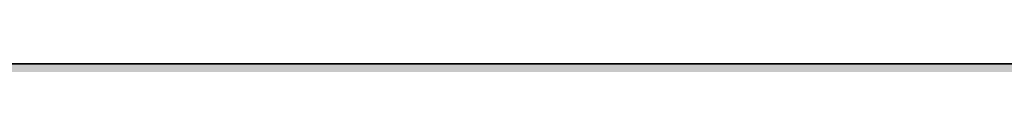
# Model space of a CAD drawing. Units: inches. Extents: x 2091 to 2899, y 967 to 2217.
# Tile 59 of 256: x 2212.20615 to 2212.29411, y 1099.91903 to 1099.91906. Entities that reach past the tile are written whole.
import ezdxf

# ---------------------------------------------------------------- set-up
doc = ezdxf.new("R2010")
doc.units = ezdxf.units.IN
doc.layers.add('A-WALL-PATT', color=141, linetype='Continuous', lineweight=13, true_color=0xadddf7)
doc.layers.add('L-SITE-WALL', color=7, linetype='Continuous', lineweight=35)

msp = doc.modelspace()

# ---------------------------------------------------------------- hatches: boundary and pattern name
at = {"layer": 'A-WALL-PATT'}
h = msp.add_hatch(color=256, dxfattribs=at)
h.dxf.hatch_style = 1
h.paths.add_polyline_path([(2212.143603, 1941.419059), (2387.643603, 1941.419059), (2387.643603, 1824.419059), (2392.143603, 1824.419059), (2392.143603, 1941.419059), (2609.643603, 1941.419059), (2609.643603, 1825.919059), (2614.143603, 1825.919059), (2614.143603, 1941.419059), (2794.143603, 1941.419059), (2794.143603, 1928.762166), (2803.143603, 1928.762166), (2803.143603, 2050.919059), (2203.143603, 2050.919059), (2203.143603, 1900.757859), (2212.143603, 1900.757859)])
h.paths.add_polyline_path([(2212.143603, 1945.919059), (2212.143603, 2041.919059), (2794.143603, 2041.919059), (2794.143603, 1945.919059), (2402.248245, 1945.919059), (2401.102434, 1945.775832), (2398.702434, 1945.775832)], flags=16)
h.paths.add_polyline_path([(2230.229861, 1948.062793), (2227.349861, 1949.502793), (2225.909861, 1951.902793), (2223.989861, 1952.862793), (2223.029861, 1955.262793), (2222.069861, 1959.582793), (2222.069861, 1963.422793), (2223.029861, 1965.662793), (2223.989861, 1965.342793), (2225.58591, 1963.860747), (2226.911533, 1964.957259), (2226.948861, 1965.938793), (2227.778319, 1966.952143), (2228.199916, 1968.878704), (2230.709861, 1964.862793), (2233.589861, 1966.302793), (2233.607309, 1966.331873), (2233.772659, 1964.938205), (2234.633802, 1963.676473), (2235.029861, 1963.902793), (2236.282035, 1965.572358), (2235.989861, 1962.942793), (2237.954512, 1957.540002), (2238.389861, 1957.902793), (2239.215861, 1960.305793), (2238.654565, 1966.38496), (2238.692792, 1966.438069), (2238.840578, 1967.499707), (2238.780291, 1967.687486), (2238.880538, 1967.786763), (2238.666861, 1966.251793), (2239.215861, 1960.305793), (2238.389861, 1957.902793), (2236.949861, 1956.702793), (2234.549861, 1949.982793)], flags=0)
h.paths.add_polyline_path([(2278.011974, 1948.062793), (2276.496427, 1947.873349), (2275.849833, 1947.688608), (2274.651974, 1947.102793)], flags=0)
h.paths.add_polyline_path([(2269.851974, 1955.742793), (2268.276176, 1956.629329), (2270.867302, 1956.348398), (2269.371974, 1958.142793), (2268.714964, 1959.192325), (2270.569833, 1958.728608), (2268.580725, 1961.906087), (2270.811974, 1960.891883), (2270.811974, 1963.422793), (2271.393315, 1964.779256), (2270.291762, 1966.156196), (2271.771974, 1965.662793), (2272.141387, 1966.524757), (2273.929833, 1965.928608), (2275.630385, 1968.054299), (2276.331938, 1966.72186), (2276.520431, 1966.952143), (2276.942029, 1968.878704), (2277.734293, 1967.611082), (2278.139888, 1969.46452), (2279.659124, 1967.033742), (2280.411974, 1966.782793), (2280.949302, 1967.588785), (2281.609833, 1967.368608), (2282.133266, 1968.153758), (2282.349235, 1966.333445), (2282.349849, 1966.332585), (2283.40755, 1968.09542), (2283.712631, 1965.52402), (2284.320221, 1964.633789), (2284.511809, 1964.889239), (2284.234974, 1965.704793), (2284.500472, 1967.318958), (2284.907944, 1965.41742), (2285.396313, 1966.068579), (2285.432833, 1966.290608), (2285.473338, 1966.171279), (2286.353919, 1967.345387), (2286.222007, 1966.158173), (2287.663492, 1968.080154), (2287.713974, 1968.442793), (2288.481599, 1969.016679), (2288.573993, 1968.728897), (2288.917461, 1969.06904), (2288.606833, 1966.837608), (2288.928726, 1963.35131), (2288.934974, 1963.356793), (2288.929731, 1963.340422), (2289.015281, 1962.413869), (2290.111223, 1963.875126), (2290.132833, 1963.942608), (2290.217672, 1964.017058), (2290.111223, 1963.875126), (2289.155833, 1960.891608), (2288.594036, 1959.257227), (2288.571974, 1959.102793), (2289.531974, 1960.542793), (2290.011974, 1962.462793), (2290.19184, 1962.642659), (2289.769833, 1959.688608), (2286.889833, 1957.288608), (2284.489833, 1950.568608), (2283.314658, 1950.046308), (2283.291974, 1949.982793), (2280.290059, 1948.648608), (2281.129833, 1948.648608), (2282.569833, 1948.168608), (2283.204726, 1948.062793), (2278.971974, 1948.062793), (2276.091974, 1949.502793), (2274.651974, 1951.902793), (2272.731974, 1952.862793)], flags=0)
h.paths.add_polyline_path([(2271.158868, 1958.021765), (2272.969833, 1955.848608), (2272.009833, 1960.168608), (2272.009833, 1964.008608), (2272.624426, 1965.442658), (2274.328023, 1963.860747), (2275.653646, 1964.957259), (2275.637743, 1964.53909), (2277.412231, 1966.006888), (2277.032974, 1965.156793), (2276.829924, 1964.975597), (2276.766012, 1963.295014), (2277.449635, 1962.66022), (2279.451974, 1964.862793), (2282.331974, 1966.302793), (2283.529833, 1966.888608), (2283.294512, 1966.770948), (2283.912993, 1963.8847), (2284.899249, 1964.448275), (2284.731974, 1962.942793), (2286.696625, 1957.540002), (2287.131974, 1957.902793), (2287.541913, 1959.095388), (2287.779395, 1958.442311), (2285.682738, 1956.695097), (2285.876503, 1959.795336), (2284.731974, 1962.942793), (2284.899249, 1964.448275), (2283.912993, 1963.8847), (2284.223833, 1962.434116), (2283.424365, 1963.605484), (2281.609833, 1962.568608), (2281.129833, 1960.168608), (2282.089833, 1956.328608), (2283.049833, 1952.968608), (2282.569833, 1950.568608), (2280.169833, 1948.648608), (2279.883316, 1948.791867), (2278.971974, 1948.062793), (2278.971974, 1949.022793), (2278.672313, 1949.397368), (2277.289833, 1950.088608), (2275.849833, 1952.488608), (2273.929833, 1953.448608), (2272.489833, 1954.888608), (2271.921647, 1954.888608), (2271.771974, 1955.262793)], flags=0)
h.paths.add_polyline_path([(2311.994146, 1955.742793), (2312.062717, 1955.674221), (2312.0551, 1955.7085)], flags=0)
h.paths.add_polyline_path([(2331.956146, 1963.951793), (2333.396146, 1965.391793), (2331.077146, 1963.356793), (2330.998603, 1963.111517)], flags=0)
h.paths.add_polyline_path([(2310.554146, 1954.302793), (2307.039807, 1956.279943), (2310.762903, 1955.876284), (2312.474146, 1953.822793), (2313.434146, 1951.422793), (2315.354146, 1950.462793), (2316.794146, 1948.062793), (2317.466146, 1947.726793), (2319.368691, 1947.964611), (2317.754146, 1949.982793), (2317.569531, 1950.610485), (2316.794146, 1951.902793), (2314.874146, 1952.862793), (2313.914146, 1955.262793), (2311.514146, 1958.142793), (2309.375489, 1961.559168), (2311.514146, 1960.337078), (2311.514146, 1961.982793), (2310.604672, 1963.119635), (2311.726605, 1962.47853), (2312.418332, 1964.09256), (2312.255964, 1964.29552), (2313.194146, 1963.982793), (2313.914146, 1965.662793), (2314.646778, 1965.418582), (2315.354146, 1966.302793), (2316.794146, 1967.742793), (2316.157435, 1966.946904), (2317.034111, 1965.28186), (2317.222604, 1965.512143), (2317.777048, 1968.045771), (2318.474111, 1966.72186), (2318.662604, 1966.952143), (2319.084201, 1968.878704), (2321.207049, 1965.482147), (2322.161419, 1966.913702), (2322.554146, 1966.782793), (2322.785988, 1967.130555), (2322.881646, 1966.324293), (2323.312041, 1965.72174), (2323.651289, 1965.891364), (2324.3965, 1967.133382), (2324.656945, 1964.938205), (2324.971986, 1964.476611), (2325.38728, 1967.001499), (2325.940813, 1964.418348), (2327.228929, 1966.135836), (2327.16632, 1965.572358), (2328.059139, 1966.762783), (2328.224576, 1966.247486), (2329.667971, 1967.67691), (2329.664576, 1967.687486), (2329.764823, 1967.786763), (2329.551146, 1966.251793), (2330.100146, 1960.305793), (2329.332814, 1958.07347), (2329.313065, 1957.935225), (2329.634146, 1958.202793), (2330.234146, 1959.102793), (2330.714146, 1961.022793), (2331.034146, 1961.342793), (2330.714146, 1959.102793), (2329.634146, 1958.202793), (2329.274146, 1957.662793), (2327.712112, 1956.361098), (2325.434146, 1949.982793), (2324.333769, 1949.493736), (2323.994146, 1948.542793), (2319.674146, 1946.622793), (2316.794146, 1948.062793), (2315.354146, 1950.462793), (2313.434146, 1951.422793)], flags=0)
h.paths.add_polyline_path([(2321.335684, 1947.952023), (2321.114146, 1948.062793), (2321.114146, 1949.022793), (2319.194146, 1951.422793), (2316.794146, 1959.582793), (2316.663237, 1959.582793), (2315.354146, 1958.142793), (2314.394146, 1958.142793), (2313.148303, 1958.709085), (2312.954146, 1959.582793), (2312.954146, 1960.891883), (2315.834146, 1959.582793), (2316.663237, 1959.582793), (2317.314709, 1960.299412), (2315.030195, 1962.420747), (2316.355818, 1963.517259), (2316.372337, 1963.951615), (2316.470195, 1963.860747), (2317.795818, 1964.957259), (2317.755219, 1963.889687), (2319.175146, 1965.156793), (2319.498407, 1965.881372), (2321.114146, 1965.342793), (2323.235885, 1962.372358), (2325.686349, 1963.772623), (2325.542789, 1962.480576), (2325.198783, 1963.494014), (2324.47851, 1963.082429), (2324.926005, 1960.994116), (2324.078087, 1962.236473), (2322.414791, 1961.286018), (2322.074146, 1959.582793), (2323.034146, 1955.742793), (2323.994146, 1952.382793), (2323.514146, 1949.982793), (2322.142717, 1948.88565), (2322.074146, 1948.542793)], flags=0)
h.paths.add_polyline_path([(2320.207479, 1963.337459), (2320.154146, 1963.422793), (2320.394146, 1963.542793)], flags=0)
h.paths.add_polyline_path([(2353.850527, 1965.8105), (2354.030527, 1965.7505), (2354.330527, 1966.4505), (2354.330527, 1966.9305)], flags=0)
h.paths.add_polyline_path([(2359.020582, 1969.026412), (2359.098382, 1968.901932), (2359.233527, 1969.5195), (2359.233527, 1969.9995)], flags=0)
h.paths.add_polyline_path([(2358.256694, 1966.681672), (2357.983601, 1966.348035), (2358.211267, 1966.146175), (2358.410492, 1966.389568)], flags=0)
h.paths.add_polyline_path([(2357.768473, 1966.058778), (2357.7322, 1965.104967), (2357.751047, 1965.120556), (2357.769527, 1965.6065), (2357.769527, 1966.057843)], flags=0)
h.paths.add_polyline_path([(2359.111527, 1965.3045), (2359.111527, 1964.8245), (2359.844527, 1966.4675), (2359.844527, 1966.9475)], flags=0)
h.paths.add_polyline_path([(2360.223684, 1966.621449), (2360.698527, 1969.3625), (2360.698527, 1969.8425), (2360.210527, 1967.0255), (2360.210527, 1966.6425)], flags=0)
h.paths.add_polyline_path([(2363.450527, 1967.8905), (2363.450527, 1968.3705), (2362.490527, 1966.9305), (2362.656045, 1966.698776)], flags=0)
h.paths.add_polyline_path([(2364.475523, 1966.078826), (2365.850527, 1968.3705), (2365.850527, 1968.8505), (2364.427975, 1966.479581)], flags=0)
h.paths.add_polyline_path([(2366.313527, 1965.8525), (2366.366709, 1965.695829), (2366.802527, 1968.3455), (2366.802527, 1968.8255)], flags=0)
h.paths.add_polyline_path([(2367.16531, 1965.803544), (2367.290527, 1966.9305), (2367.290527, 1967.4105), (2367.102701, 1965.720066)], flags=0)
h.paths.add_polyline_path([(2370.036527, 1959.9735), (2371.013527, 1963.0245), (2371.013527, 1963.5045), (2370.036527, 1960.4535)], flags=0)
h.paths.add_polyline_path([(2371.610527, 1960.2105), (2372.570527, 1961.6505), (2372.570527, 1962.1305), (2371.802527, 1960.9785)], flags=0)
h.paths.add_polyline_path([(2350.873666, 1956.005086), (2351.930527, 1955.8905), (2354.490527, 1953.3305), (2353.850527, 1954.9305), (2351.450527, 1957.8105), (2347.935527, 1963.4255), (2347.935527, 1963.9055), (2351.450527, 1958.2905), (2353.705073, 1955.585046), (2352.890527, 1959.2505), (2352.890527, 1959.7305), (2352.890527, 1961.924786), (2356.730527, 1959.7305), (2358.454471, 1961.626838), (2354.810527, 1965.0105), (2355.030855, 1965.28591), (2358.691091, 1961.88712), (2361.530527, 1965.0105), (2364.376495, 1966.433484), (2364.524394, 1965.186911), (2365.454468, 1963.824181), (2365.881073, 1964.067955), (2365.370527, 1966.4505), (2365.370527, 1966.9305), (2366.810527, 1960.2105), (2366.810527, 1959.7305), (2366.388709, 1952.981409), (2367.770527, 1956.8505), (2368.641225, 1957.576082), (2366.810527, 1962.6105), (2366.810527, 1963.0905), (2368.775179, 1957.68771), (2369.210527, 1958.0505), (2370.001592, 1960.351867), (2369.475232, 1966.052668), (2369.513458, 1966.105777), (2369.514173, 1966.110912), (2369.475232, 1966.532668), (2369.513458, 1966.585777), (2369.614635, 1967.312591), (2369.182527, 1968.6585), (2369.182527, 1969.1385), (2369.600957, 1967.835194), (2369.701204, 1967.934471), (2369.717947, 1968.054743), (2370.145176, 1968.374145), (2369.778707, 1968.011224), (2369.701204, 1967.454471), (2370.468161, 1968.214004), (2369.674936, 1967.265771), (2369.514173, 1966.110912), (2370.036527, 1960.4535), (2370.036527, 1959.9735), (2369.441756, 1958.243191), (2370.650527, 1959.2505), (2371.045821, 1962.017559), (2371.130527, 1962.1305), (2370.650527, 1958.7705), (2367.770527, 1956.3705), (2365.370527, 1949.6505), (2362.079099, 1948.187643), (2363.450527, 1947.7305), (2361.050527, 1947.7305), (2360.090527, 1947.7305), (2357.103861, 1947.357167), (2360.090527, 1948.2105), (2358.170527, 1949.1705), (2356.730527, 1951.5705), (2354.810527, 1952.5305), (2351.930527, 1955.4105)], flags=0)
h.paths.add_polyline_path([(2361.050527, 1948.6905), (2359.130527, 1951.0905), (2356.730527, 1959.2505), (2355.770527, 1959.2505), (2352.890527, 1960.559591), (2352.890527, 1961.444786), (2355.890527, 1959.7305), (2356.730527, 1959.7305), (2356.837194, 1959.367834), (2361.530527, 1964.5305), (2363.248422, 1965.389448), (2364.92531, 1963.041805), (2362.490527, 1961.6505), (2362.063861, 1959.517167), (2362.970527, 1955.8905), (2363.930527, 1952.5305), (2363.930527, 1952.0505), (2363.450527, 1949.6505), (2361.050527, 1947.7305)], flags=0)
h.paths.add_polyline_path([(2359.130527, 1951.5705), (2359.290527, 1951.3705), (2361.050527, 1954.4505), (2361.050527, 1954.9305)], flags=0)
h.paths.add_polyline_path([(2357.219527, 1966.5455), (2356.792527, 1968.8145), (2356.792527, 1969.2945), (2357.219527, 1967.0255)], flags=0)
h.paths.add_polyline_path([(2361.050527, 1954.4505), (2361.530527, 1958.7705), (2361.530527, 1959.2505), (2361.050527, 1954.9305)], flags=0)
h.paths.add_polyline_path([(2402.548287, 1948.486076), (2402.302434, 1948.415832), (2402.590434, 1948.415832)], flags=0)
h.paths.add_polyline_path([(2394.142434, 1956.095832), (2395.685052, 1954.553214), (2396.720495, 1953.970679), (2396.062434, 1955.615832), (2395.241381, 1956.601096), (2395.878904, 1956.441715), (2395.102434, 1959.935832), (2395.102434, 1963.775832), (2396.062434, 1966.015832), (2397.022434, 1965.695832), (2398.618483, 1964.213787), (2399.944106, 1965.310299), (2399.981434, 1966.291832), (2400.810891, 1967.305183), (2401.232489, 1969.231744), (2403.537949, 1965.543008), (2403.941984, 1967.389316), (2404.702434, 1967.135832), (2405.460328, 1966.07478), (2406.622434, 1966.655832), (2406.639882, 1966.684913), (2406.805232, 1965.291245), (2406.925694, 1965.114746), (2407.342434, 1964.975832), (2407.874326, 1965.77367), (2408.1691, 1964.398055), (2409.314608, 1965.925398), (2409.217458, 1965.051054), (2409.445232, 1963.131245), (2410.306374, 1961.869513), (2410.702434, 1962.095832), (2411.442269, 1963.082279), (2411.165434, 1963.897832), (2411.616426, 1966.639757), (2411.725365, 1966.791109), (2411.873151, 1967.852747), (2411.812864, 1968.040526), (2411.913111, 1968.139803), (2411.699434, 1966.604832), (2412.248434, 1960.658832), (2413.225434, 1963.709832), (2414.3779, 1964.72116), (2414.513151, 1965.692747), (2414.452864, 1965.880526), (2414.553111, 1965.979803), (2414.3779, 1964.72116), (2414.519817, 1964.845697), (2414.365365, 1964.631109), (2414.339434, 1964.444832), (2414.888434, 1958.498832), (2414.062434, 1956.095832), (2412.622434, 1954.895832), (2410.17137, 1948.032854), (2410.016719, 1948.084404), (2405.902434, 1946.255832), (2405.902434, 1947.215832), (2405.204252, 1948.08856), (2404.222434, 1948.415832), (2403.262434, 1948.415832), (2400.382434, 1949.855832), (2399.662434, 1951.055832), (2397.982434, 1952.735832), (2397.022434, 1953.215832), (2395.685052, 1954.553214), (2392.656776, 1956.256908)], flags=0)
h.paths.add_polyline_path([(2409.08565, 1964.407441), (2409.130363, 1964.275715), (2409.262434, 1964.495832)], flags=0)
h.paths.add_polyline_path([(2397.742434, 1961.615832), (2398.702434, 1963.855832), (2399.662434, 1963.535832), (2401.426563, 1965.740994), (2401.791415, 1966.5588), (2402.071434, 1965.070832), (2402.835507, 1964.393367), (2403.262398, 1964.9149), (2403.338119, 1964.771086), (2402.615516, 1963.976223), (2402.498612, 1960.902238), (2403.542997, 1959.932452), (2404.413203, 1960.889679), (2404.702434, 1962.335832), (2407.916347, 1964.172354), (2409.520211, 1961.926944), (2410.987085, 1957.893042), (2411.422434, 1958.255832), (2412.047964, 1960.075625), (2412.410341, 1959.079088), (2411.675621, 1958.466821), (2411.662434, 1958.255832), (2411.62607, 1958.425529), (2409.982434, 1957.055832), (2407.582434, 1950.335832), (2403.262434, 1948.415832), (2403.262434, 1949.375832), (2401.342434, 1951.775832), (2399.416508, 1958.323981), (2397.742434, 1959.084923), (2397.742434, 1959.970118), (2397.102434, 1960.335832), (2397.742434, 1960.044923)], flags=0)
h.paths.add_polyline_path([(2405.902434, 1952.975832), (2405.950434, 1953.407832), (2406.016719, 1953.175832)], flags=0)
h.paths.add_polyline_path([(2449.817778, 1967.114014), (2449.752323, 1967.135832), (2449.793703, 1967.077901)], flags=0)
h.paths.add_polyline_path([(2451.697696, 1966.61812), (2451.740895, 1966.690118), (2451.692051, 1966.665696)], flags=0)
h.paths.add_polyline_path([(2454.343628, 1965.737572), (2455.752323, 1967.615832), (2455.992323, 1968.095832), (2454.364497, 1965.925398)], flags=0)
h.paths.add_polyline_path([(2457.547323, 1968.863832), (2457.787323, 1969.343832), (2457.054323, 1968.795832), (2457.007622, 1968.460345)], flags=0)
h.paths.add_polyline_path([(2456.921784, 1967.856662), (2456.802238, 1968.229016), (2456.723, 1967.659803)], flags=0)
h.paths.add_polyline_path([(2457.302323, 1967.376832), (2457.542323, 1967.856832), (2456.810323, 1966.839832), (2456.740516, 1966.700218), (2456.749021, 1966.608105)], flags=0)
h.paths.add_polyline_path([(2458.275323, 1963.709832), (2458.155343, 1963.335153), (2460.354323, 1965.264832), (2460.594323, 1965.744832)], flags=0)
h.paths.add_polyline_path([(2458.392323, 1962.815832), (2458.364088, 1962.618185), (2459.592323, 1964.255832), (2459.832323, 1964.735832)], flags=0)
h.paths.add_polyline_path([(2459.352323, 1962.815832), (2459.272323, 1962.495832), (2460.072323, 1963.295832), (2460.312323, 1963.775832)], flags=0)
h.paths.add_polyline_path([(2458.680323, 1960.607832), (2458.632323, 1960.415832), (2459.592323, 1961.855832), (2459.832323, 1962.335832)], flags=0)
h.paths.add_polyline_path([(2437.83817, 1956.24265), (2439.192323, 1956.095832), (2441.352323, 1953.935832), (2440.872323, 1955.135832), (2438.472323, 1958.015832), (2438.071563, 1958.656023), (2438.712323, 1958.495832), (2440.639596, 1956.183105), (2439.912323, 1959.455832), (2439.912323, 1963.295832), (2441.352323, 1966.655832), (2441.592323, 1967.135832), (2441.112323, 1966.015832), (2442.072323, 1965.695832), (2443.988993, 1968.09167), (2444.241323, 1966.750832), (2444.916801, 1966.15192), (2445.676574, 1967.080136), (2446.255323, 1969.724832), (2446.495323, 1970.204832), (2446.282379, 1969.231744), (2447.362672, 1967.503275), (2447.720323, 1969.567832), (2447.960323, 1970.047832), (2447.48548, 1967.306781), (2448.792323, 1965.215832), (2448.472323, 1964.863832), (2448.552323, 1964.735832), (2451.452051, 1966.185696), (2451.615122, 1964.811245), (2452.307917, 1963.796172), (2453.234505, 1964.325651), (2454.072323, 1960.415832), (2453.628687, 1953.317651), (2454.792323, 1956.575832), (2455.032323, 1957.055832), (2455.718835, 1957.627926), (2453.832323, 1962.815832), (2453.940966, 1963.793615), (2453.335323, 1965.577832), (2453.824323, 1968.550832), (2454.064323, 1969.030832), (2453.575323, 1966.057832), (2454.040333, 1964.687919), (2453.832323, 1962.815832), (2455.718835, 1957.627926), (2456.367207, 1958.168235), (2457.058323, 1960.178832), (2457.298323, 1960.658832), (2456.472323, 1958.255832), (2457.717729, 1959.29367), (2457.672323, 1958.975832), (2454.889951, 1956.657188), (2453.614142, 1953.084923), (2453.592323, 1952.735832), (2453.352323, 1952.255832), (2453.359596, 1952.372196), (2452.632323, 1950.335832), (2452.392323, 1949.855832), (2449.203752, 1948.43869), (2450.712323, 1947.935832), (2448.072323, 1947.935832), (2447.112323, 1947.935832), (2444.552323, 1947.615832), (2447.199596, 1948.372196), (2445.192323, 1949.375832), (2443.752323, 1951.775832), (2441.832323, 1952.735832), (2438.952323, 1955.615832)], flags=0)
h.paths.add_polyline_path([(2443.992323, 1959.935832), (2444.040323, 1959.772632), (2444.121554, 1959.861986)], flags=0)
h.paths.add_polyline_path([(2442.912323, 1959.935832), (2443.032323, 1959.935832), (2442.445657, 1960.202499)], flags=0)
h.paths.add_polyline_path([(2444.982943, 1965.019677), (2445.279323, 1965.264832), (2445.519323, 1965.744832), (2444.993996, 1965.310299)], flags=0)
h.paths.add_polyline_path([(2446.133323, 1965.029832), (2446.330366, 1965.471499), (2444.970323, 1964.257832), (2444.730323, 1963.777832)], flags=0)
h.paths.add_polyline_path([(2442.792323, 1959.455832), (2443.752323, 1959.455832), (2446.152323, 1951.295832), (2446.412323, 1951.750832), (2446.392323, 1951.775832), (2448.080599, 1954.730315), (2448.552323, 1958.975832), (2441.832323, 1965.215832), (2442.154946, 1965.619111), (2448.792323, 1959.455832), (2448.312323, 1955.135832), (2448.072323, 1954.655832), (2446.412323, 1951.750832), (2448.312323, 1949.375832), (2448.312323, 1948.415832), (2450.540895, 1950.19869), (2450.952323, 1952.255832), (2449.992323, 1955.615832), (2449.032323, 1959.455832), (2449.512323, 1961.855832), (2449.752323, 1962.335832), (2449.674904, 1961.948736), (2452.994505, 1963.845651), (2453.064414, 1963.519409), (2452.884611, 1963.782854), (2449.674904, 1961.948736), (2449.272323, 1959.935832), (2450.232323, 1956.095832), (2451.192323, 1952.735832), (2450.712323, 1950.335832), (2450.472323, 1949.855832), (2448.072323, 1947.935832), (2448.072323, 1948.535832), (2445.432323, 1949.855832), (2443.992323, 1952.255832), (2442.072323, 1953.215832), (2441.112323, 1955.615832), (2440.152323, 1959.935832), (2440.152323, 1960.655832)], flags=0)
h.paths.add_polyline_path([(2456.692323, 1966.985832), (2457.608323, 1968.080832), (2457.848323, 1968.560832), (2456.932323, 1967.465832)], flags=0)
h.paths.add_polyline_path([(2489.89657, 1966.580241), (2489.942948, 1966.189347), (2490.747488, 1967.530248), (2491.319122, 1968.951161)], flags=0)
h.paths.add_polyline_path([(2473.562471, 1956.407131), (2477.139981, 1956.019257), (2476.955333, 1956.240834), (2475.108049, 1957.280108), (2476.347488, 1956.970248), (2475.186901, 1958.824216), (2476.919122, 1958.391161), (2475.411642, 1960.799269), (2477.787488, 1959.719339), (2477.787488, 1962.250248), (2477.637399, 1962.43786), (2477.82255, 1962.332059), (2478.359122, 1963.58406), (2478.359122, 1963.671161), (2477.324348, 1964.964628), (2478.714826, 1964.501135), (2479.319122, 1965.911161), (2480.279122, 1965.591161), (2481.783965, 1967.472214), (2482.116488, 1965.705248), (2482.880562, 1965.027782), (2483.209305, 1965.429408), (2483.220169, 1965.71509), (2483.07594, 1965.989022), (2483.711762, 1966.765808), (2484.130488, 1968.679248), (2484.702122, 1970.100161), (2484.489177, 1969.127072), (2486.502904, 1965.905109), (2487.387488, 1965.610248), (2488.153419, 1966.759144), (2488.717017, 1965.970108), (2489.200086, 1966.211642), (2489.330671, 1965.110992), (2490.393905, 1963.622465), (2490.660765, 1963.774956), (2490.493905, 1964.553636), (2490.923063, 1963.924841), (2491.319122, 1964.151161), (2491.333389, 1964.170183), (2491.210488, 1964.532248), (2491.281756, 1964.965537), (2491.425789, 1964.293383), (2494.076476, 1967.827632), (2494.497918, 1966.514942), (2494.598165, 1966.614218), (2494.689488, 1967.270248), (2495.106748, 1967.582196), (2495.129839, 1967.748075), (2495.069552, 1967.935854), (2495.169799, 1968.035131), (2495.031777, 1967.043632), (2495.753818, 1967.758684), (2494.982053, 1966.686437), (2494.956122, 1966.500161), (2495.479021, 1960.836851), (2495.910488, 1962.184248), (2496.482122, 1963.605161), (2496.072694, 1962.326589), (2496.768904, 1962.937536), (2496.599122, 1962.711161), (2496.119122, 1959.351161), (2496.732873, 1960.271787), (2496.987488, 1961.290248), (2497.559122, 1962.711161), (2497.079122, 1960.791161), (2496.507488, 1959.370248), (2495.547488, 1957.930248), (2492.758842, 1955.606376), (2490.839122, 1950.231161), (2490.267488, 1948.810248), (2485.947488, 1946.890248), (2483.067488, 1948.330248), (2481.627488, 1950.730248), (2479.707488, 1951.690248), (2476.827488, 1954.570248)], flags=0)
h.paths.add_polyline_path([(2485.576973, 1948.313392), (2485.559122, 1948.311161), (2485.578758, 1948.311161)], flags=0)
h.paths.add_polyline_path([(2478.645063, 1954.551161), (2478.109042, 1956.963257), (2479.319122, 1955.511161), (2480.279122, 1953.111161), (2482.199122, 1952.151161), (2483.639122, 1949.751161), (2486.519122, 1948.311161), (2486.519122, 1949.271161), (2484.739307, 1951.49593), (2484.027488, 1950.250248), (2481.627488, 1958.410248), (2482.375148, 1959.232673), (2482.199122, 1959.831161), (2483.197572, 1960.929456), (2479.707488, 1964.170248), (2480.603358, 1965.290085), (2481.875171, 1964.109115), (2482.666387, 1964.763582), (2482.615359, 1963.421798), (2482.989199, 1963.074661), (2484.008488, 1963.984248), (2484.683606, 1965.497507), (2484.580122, 1965.405161), (2485.357268, 1967.147113), (2485.120645, 1965.781197), (2486.427488, 1963.690248), (2488.145383, 1964.549195), (2489.822271, 1962.201552), (2490.747488, 1962.730248), (2491.999662, 1964.399813), (2492.076046, 1965.087265), (2492.212892, 1964.684119), (2492.485374, 1965.047429), (2492.279122, 1963.191161), (2494.243773, 1957.78837), (2494.562503, 1958.053978), (2494.933488, 1959.133248), (2495.505122, 1960.554161), (2494.679122, 1958.151161), (2494.107488, 1956.730248), (2494.562503, 1958.053978), (2493.408544, 1957.092345), (2491.707488, 1961.770248), (2491.999662, 1964.399813), (2490.747488, 1962.730248), (2487.71203, 1960.9957), (2487.479122, 1959.831161), (2488.439122, 1955.991161), (2489.399122, 1952.631161), (2488.919122, 1950.231161), (2488.576918, 1949.957397), (2488.347488, 1948.810248), (2487.651715, 1948.253629), (2487.479122, 1948.311161), (2486.519122, 1948.311161), (2483.639122, 1949.751161), (2482.199122, 1952.151161), (2480.279122, 1953.111161), (2478.839122, 1954.551161)], flags=0)
h.paths.add_polyline_path([(2526.648252, 1966.987524), (2526.517343, 1967.031161), (2526.600102, 1966.915298)], flags=0)
h.paths.add_polyline_path([(2528.47064, 1966.446656), (2528.574486, 1966.619732), (2528.457071, 1966.561025)], flags=0)
h.paths.add_polyline_path([(2534.133343, 1967.496161), (2534.156685, 1967.542845), (2534.059841, 1967.408296)], flags=0)
h.paths.add_polyline_path([(2536.161923, 1964.0506), (2535.157343, 1962.711161), (2535.100872, 1962.315866), (2536.117343, 1963.671161), (2536.420532, 1964.277539)], flags=0)
h.paths.add_polyline_path([(2535.157343, 1959.831161), (2536.117343, 1961.271161), (2536.597343, 1962.231161), (2535.253343, 1960.215161)], flags=0)
h.paths.add_polyline_path([(2513.249035, 1956.284796), (2516.221181, 1955.962555), (2514.997343, 1957.431161), (2514.195823, 1958.711541), (2515.477343, 1958.391161), (2516.931888, 1956.645706), (2516.437343, 1958.871161), (2516.437343, 1962.711161), (2516.872692, 1963.726974), (2515.346434, 1965.634797), (2517.397343, 1964.951161), (2517.877343, 1966.071161), (2518.357343, 1967.031161), (2517.877343, 1965.911161), (2518.837343, 1965.591161), (2520.48659, 1967.652719), (2520.766343, 1966.166161), (2521.530417, 1965.488695), (2521.781443, 1965.795375), (2521.800911, 1966.307268), (2521.477804, 1966.920936), (2521.246343, 1967.126161), (2521.177701, 1967.490913), (2521.477804, 1966.920936), (2522.010417, 1966.448695), (2522.257386, 1966.750417), (2522.780343, 1969.140161), (2523.260343, 1970.100161), (2523.047398, 1969.127072), (2524.673132, 1966.525897), (2526.037343, 1966.071161), (2526.795238, 1965.010108), (2527.977071, 1965.601025), (2528.140141, 1964.226573), (2528.66459, 1963.458159), (2529.388616, 1963.871888), (2529.329665, 1964.14699), (2529.481284, 1963.924841), (2529.877343, 1964.151161), (2529.98401, 1964.293383), (2529.789053, 1965.20318), (2530.0624, 1964.397903), (2532.802483, 1968.051347), (2533.147773, 1966.975854), (2533.24802, 1967.075131), (2533.339343, 1967.731161), (2533.672848, 1967.980493), (2533.72802, 1968.035131), (2533.514343, 1966.500161), (2534.024718, 1960.972496), (2534.560343, 1962.645161), (2535.040343, 1963.605161), (2534.063343, 1960.554161), (2533.237343, 1958.151161), (2534.288154, 1959.026836), (2534.197343, 1958.391161), (2531.512597, 1956.153872), (2529.397343, 1950.231161), (2528.917343, 1949.271161), (2526.448772, 1948.174018), (2527.477343, 1947.831161), (2530.357343, 1947.351161), (2524.597343, 1947.351161), (2521.717343, 1948.791161), (2520.277343, 1951.191161), (2518.357343, 1952.151161), (2515.477343, 1955.031161)], flags=0)
h.paths.add_polyline_path([(2523.93476, 1967.190308), (2523.619512, 1966.483689), (2523.7705, 1966.242109)], flags=0)
h.paths.add_polyline_path([(2518.837343, 1953.111161), (2517.877343, 1955.511161), (2516.884983, 1959.976779), (2516.917343, 1959.96207), (2516.917343, 1962.025446), (2520.757343, 1959.831161), (2522.024949, 1961.225527), (2518.357343, 1964.631161), (2519.002589, 1965.437718), (2520.433392, 1964.109115), (2521.30112, 1964.826871), (2521.245157, 1963.355333), (2525.638307, 1959.27598), (2526.037343, 1961.271161), (2529.397343, 1963.191161), (2530.649517, 1964.860726), (2530.66472, 1964.99755), (2530.691956, 1964.917311), (2531.087778, 1965.445074), (2530.945985, 1964.168944), (2530.691956, 1964.917311), (2529.397343, 1963.191161), (2526.362504, 1961.456967), (2526.037343, 1959.831161), (2526.997343, 1955.991161), (2527.957343, 1952.631161), (2527.477343, 1950.231161), (2527.134486, 1949.956875), (2526.973928, 1949.154087), (2526.697343, 1949.031161), (2524.597343, 1947.351161), (2524.597343, 1948.311161), (2524.277343, 1948.711161), (2522.197343, 1949.751161), (2520.757343, 1952.151161)], flags=0)
h.paths.add_polyline_path([(2520.277343, 1958.871161), (2520.853343, 1959.504761), (2523.157343, 1951.671161), (2524.613895, 1954.220126), (2524.597343, 1954.071161), (2522.677343, 1950.711161)], flags=0)
h.paths.add_polyline_path([(2559.37091, 1966.311161), (2559.398411, 1966.324911), (2559.401943, 1966.345296)], flags=0)
h.paths.add_polyline_path([(2549.77091, 1957.191161), (2552.65091, 1954.311161), (2552.133987, 1955.603468), (2550.61091, 1957.431161), (2547.09591, 1963.046161), (2545.77591, 1965.206161), (2549.29091, 1959.591161), (2551.69091, 1956.711161), (2550.792933, 1960.752059), (2550.73091, 1960.780251), (2550.73091, 1964.871161), (2551.69091, 1967.111161), (2552.65091, 1966.791161), (2554.246959, 1965.309115), (2555.034252, 1965.960337), (2555.581671, 1966.644612), (2555.60991, 1967.387161), (2556.439368, 1968.400511), (2556.860966, 1970.327072), (2559.37091, 1966.311161), (2560.69091, 1964.151161), (2562.408805, 1965.010108), (2561.65091, 1966.071161), (2560.33091, 1968.231161), (2561.758497, 1966.23254), (2562.347213, 1967.115614), (2562.433709, 1966.386573), (2563.127798, 1965.369604), (2563.57091, 1965.591161), (2563.588359, 1965.620241), (2563.362543, 1967.52354), (2563.722489, 1965.843792), (2565.060001, 1968.072979), (2564.732862, 1965.128722), (2565.117577, 1963.333383), (2567.444622, 1966.436109), (2567.315615, 1967.833328), (2567.353841, 1967.886437), (2567.501627, 1968.948075), (2567.44134, 1969.135854), (2567.541587, 1969.235131), (2567.32791, 1967.700161), (2567.87691, 1961.754161), (2568.746689, 1964.470327), (2568.635615, 1965.673328), (2568.673841, 1965.726437), (2568.821627, 1966.788075), (2568.76134, 1966.975854), (2568.861587, 1967.075131), (2568.64791, 1965.540161), (2568.726127, 1964.693026), (2568.85391, 1964.805161), (2568.746689, 1964.470327), (2568.817236, 1963.706261), (2568.97091, 1963.911161), (2568.866075, 1963.17731), (2569.19691, 1959.594161), (2568.37091, 1957.191161), (2566.93091, 1955.991161), (2564.620272, 1949.521373), (2564.65091, 1949.511161), (2564.616625, 1949.511161), (2564.53091, 1949.271161), (2560.21091, 1947.351161), (2557.33091, 1948.791161), (2556.045196, 1950.934018), (2556.01091, 1950.951161), (2555.856625, 1951.208303), (2553.97091, 1952.151161), (2551.09091, 1955.031161), (2546.650144, 1957.529515)], flags=0)
h.paths.add_polyline_path([(2567.025794, 1959.33023), (2567.035007, 1959.304895), (2567.05091, 1959.351161)], flags=0)
h.paths.add_polyline_path([(2551.968287, 1962.518374), (2553.01091, 1964.951161), (2553.97091, 1964.631161), (2555.566959, 1963.149115), (2556.892583, 1964.245627), (2556.92991, 1965.227161), (2557.143984, 1965.488695), (2556.420066, 1966.130557), (2556.391421, 1966.104995), (2556.37991, 1966.166161), (2556.420066, 1966.130557), (2556.95191, 1966.605161), (2557.092139, 1966.919478), (2557.570875, 1966.010228), (2557.759368, 1966.240511), (2557.41791, 1964.680161), (2556.892583, 1964.245627), (2556.807089, 1961.997566), (2560.69091, 1958.391161), (2560.635526, 1957.892699), (2560.81091, 1957.191161), (2561.77091, 1953.831161), (2561.29091, 1951.431161), (2559.110423, 1949.68677), (2559.156484, 1949.629193), (2563.02652, 1951.349209), (2562.61091, 1949.271161), (2560.21091, 1947.351161), (2560.21091, 1948.311161), (2559.25091, 1949.511161), (2558.89091, 1949.511161), (2558.89091, 1949.961161), (2558.29091, 1950.711161), (2558.053701, 1951.517672), (2556.97091, 1952.871161), (2555.06788, 1959.341464), (2552.05091, 1961.065446), (2552.05091, 1962.471161)], flags=0)
h.paths.add_polyline_path([(2588.330049, 1958.391161), (2588.610248, 1958.110962), (2588.553362, 1958.366949)], flags=0)
h.paths.add_polyline_path([(2594.745454, 1950.493086), (2593.957532, 1953.172022), (2593.130049, 1954.551161), (2591.210049, 1955.511161), (2590.250049, 1957.911161), (2588.309033, 1960.240379), (2586.177306, 1961.209346), (2587.850049, 1960.791161), (2587.253416, 1961.744246), (2588.441314, 1961.065446), (2588.441314, 1962.655528), (2588.421679, 1962.665345), (2588.441314, 1962.711161), (2586.914038, 1964.620256), (2588.877086, 1963.727962), (2589.290049, 1964.69154), (2589.290049, 1966.071161), (2590.250049, 1968.311161), (2591.210049, 1967.991161), (2592.806098, 1966.509115), (2594.131721, 1967.605627), (2594.169049, 1968.587161), (2594.998506, 1969.600511), (2595.420104, 1971.527072), (2597.930049, 1967.511161), (2600.810049, 1968.951161), (2600.827497, 1968.980241), (2600.992847, 1967.586573), (2601.853989, 1966.324841), (2602.107143, 1966.4695), (2602.236354, 1967.255069), (2602.356715, 1966.693383), (2603.502223, 1968.220726), (2603.210049, 1965.591161), (2605.1747, 1960.18837), (2605.506891, 1960.465196), (2605.026019, 1965.673328), (2605.064245, 1965.726437), (2605.212031, 1966.788075), (2605.151744, 1966.975854), (2605.251991, 1967.075131), (2605.343314, 1967.731161), (2605.952905, 1968.186898), (2605.874753, 1969.033328), (2605.912979, 1969.086437), (2606.060766, 1970.148075), (2606.000479, 1970.335854), (2606.100725, 1970.435131), (2605.887049, 1968.900161), (2606.436049, 1962.954161), (2605.610049, 1960.551161), (2605.997036, 1960.87365), (2606.564314, 1962.645161), (2608.241494, 1964.116941), (2608.010049, 1963.191161), (2607.050049, 1961.751161), (2606.631486, 1961.402358), (2606.201314, 1958.391161), (2603.321314, 1955.991161), (2600.921314, 1949.271161), (2596.601314, 1947.351161), (2593.721314, 1948.791161), (2592.857314, 1950.231161), (2592.650049, 1950.231161)], flags=0)
h.paths.add_polyline_path([(2596.601314, 1947.351161), (2596.601314, 1948.311161), (2594.681314, 1950.711161), (2596.154954, 1953.290029), (2595.530049, 1954.071161), (2593.199226, 1961.995957), (2592.65134, 1962.504708), (2591.780151, 1963.002531), (2593.282987, 1964.245627), (2593.320314, 1965.227161), (2594.149772, 1966.240511), (2594.57137, 1968.167072), (2596.182651, 1965.589023), (2596.951273, 1966.434508), (2598.041314, 1966.071161), (2598.799209, 1965.010108), (2599.961314, 1965.591161), (2599.978763, 1965.620241), (2600.144113, 1964.226573), (2601.005255, 1962.964841), (2601.401314, 1963.191161), (2602.653488, 1964.860726), (2602.361314, 1962.231161), (2603.792748, 1958.294719), (2601.977644, 1953.212427), (2601.946208, 1952.709453), (2599.468755, 1951.608363), (2599.001314, 1949.271161)], flags=0)
h.paths.add_polyline_path([(2597.561314, 1958.871161), (2597.670966, 1959.419419), (2597.595054, 1958.736204)], flags=0)
h.paths.add_polyline_path([(2623.666305, 1961.254375), (2625.519163, 1960.791161), (2624.965544, 1961.675533), (2627.199163, 1960.660251), (2627.199163, 1961.151161), (2626.959163, 1962.231161), (2626.959163, 1963.491161), (2625.582321, 1965.212213), (2626.959163, 1964.425446), (2626.959163, 1965.831161), (2626.869163, 1965.861161), (2627.919163, 1968.311161), (2628.879163, 1967.991161), (2630.475212, 1966.509115), (2631.800835, 1967.605627), (2631.838163, 1968.587161), (2632.667621, 1969.600511), (2633.089218, 1971.527072), (2635.599163, 1967.511161), (2638.479163, 1968.951161), (2638.496611, 1968.980241), (2638.661961, 1967.586573), (2639.176273, 1966.833011), (2639.780216, 1967.839582), (2640.02583, 1966.693383), (2641.171337, 1968.220726), (2640.879163, 1965.591161), (2641.114265, 1964.94463), (2641.411337, 1965.340726), (2641.308099, 1964.411586), (2642.843814, 1960.18837), (2643.279163, 1960.551161), (2644.084736, 1962.894736), (2643.783867, 1966.153328), (2643.806834, 1966.185237), (2643.600676, 1968.418053), (2643.522812, 1968.660581), (2643.72988, 1970.148075), (2643.669593, 1970.335854), (2643.76984, 1970.435131), (2643.556163, 1968.900161), (2643.600676, 1968.418053), (2643.909593, 1967.455854), (2644.00984, 1967.555131), (2643.811743, 1966.132079), (2644.105163, 1962.954161), (2644.238773, 1961.350836), (2644.719163, 1961.751161), (2645.032853, 1962.221695), (2645.322163, 1963.125161), (2646.07642, 1963.787047), (2645.032853, 1962.221695), (2644.345163, 1960.074161), (2643.519163, 1957.671161), (2642.079163, 1956.471161), (2639.719612, 1949.864419), (2639.875527, 1949.838433), (2635.359163, 1947.831161), (2632.479163, 1949.271161), (2631.039163, 1951.671161), (2629.119163, 1952.631161), (2628.159163, 1955.031161), (2625.759163, 1957.911161)], flags=0)
h.paths.add_polyline_path([(2627.816306, 1956.574018), (2627.373708, 1958.565706), (2626.376306, 1959.762589), (2627.199163, 1959.351161), (2627.373708, 1958.565706), (2627.919163, 1957.911161), (2628.879163, 1955.511161), (2630.799163, 1954.551161), (2632.239163, 1952.151161), (2633.315025, 1951.613229), (2631.039163, 1959.351161), (2631.49783, 1959.855694), (2630.799163, 1962.231161), (2631.449867, 1962.946935), (2630.715212, 1963.629115), (2632.040835, 1964.725627), (2632.078163, 1965.707161), (2632.292237, 1965.968695), (2631.705339, 1966.489067), (2633.136441, 1967.766144), (2633.329218, 1968.647072), (2634.674718, 1966.494272), (2635.208465, 1967.081393), (2636.799163, 1966.551161), (2637.676404, 1967.867023), (2638.993946, 1966.022465), (2639.705345, 1966.428979), (2641.119163, 1959.831161), (2640.930072, 1956.805706), (2639.439163, 1952.631161), (2638.227456, 1952.092624), (2637.759163, 1949.751161), (2635.359163, 1947.831161), (2635.359163, 1948.791161), (2633.439163, 1951.191161), (2633.315025, 1951.613229), (2632.239163, 1952.151161), (2630.799163, 1954.551161), (2628.879163, 1955.511161)], flags=0)
h.paths.add_polyline_path([(2637.759163, 1953.831161), (2637.279163, 1955.511161), (2636.319163, 1959.351161), (2636.799163, 1961.751161), (2639.233946, 1963.142465), (2637.557058, 1965.490108), (2638.738891, 1966.081025), (2638.901961, 1964.706573), (2639.763104, 1963.444841), (2636.799163, 1961.751161), (2636.532496, 1960.417827), (2637.039163, 1958.391161), (2637.999163, 1955.031161)], flags=0)
h.paths.add_polyline_path([(2668.567407, 1951.431161), (2667.607407, 1953.831161), (2665.207407, 1956.711161), (2662.293903, 1961.365307), (2665.447407, 1959.591161), (2666.647407, 1958.391161), (2666.647407, 1959.975161), (2666.058317, 1960.68207), (2666.647407, 1960.345446), (2666.647407, 1961.991161), (2666.70009, 1962.114087), (2666.407407, 1963.431161), (2666.407407, 1967.271161), (2667.367407, 1969.511161), (2668.327407, 1969.191161), (2669.923457, 1967.709115), (2671.24908, 1968.805627), (2671.286407, 1969.787161), (2672.115865, 1970.800511), (2672.537463, 1972.727072), (2675.047407, 1968.711161), (2677.927407, 1970.151161), (2677.944856, 1970.180241), (2678.110206, 1968.786573), (2678.971348, 1967.524841), (2679.367407, 1967.751161), (2680.619581, 1969.420726), (2680.327407, 1966.791161), (2682.292059, 1961.38837), (2682.727407, 1961.751161), (2683.358306, 1963.586571), (2683.232112, 1964.953328), (2683.270338, 1965.006437), (2683.393215, 1965.889138), (2683.359969, 1966.249215), (2683.357837, 1966.255854), (2683.359229, 1966.257232), (2682.992112, 1970.233328), (2683.030338, 1970.286437), (2683.178124, 1971.348075), (2683.117837, 1971.535854), (2683.218084, 1971.635131), (2683.004407, 1970.100161), (2683.359229, 1966.257232), (2683.458084, 1966.355131), (2683.393215, 1965.889138), (2683.413908, 1965.665023), (2684.42381, 1966.872275), (2683.553407, 1964.154161), (2683.358306, 1963.586571), (2683.793407, 1958.874161), (2682.967407, 1956.471161), (2681.527407, 1955.271161), (2680.109226, 1951.300251), (2680.084933, 1950.911573), (2679.976846, 1950.929587), (2679.127407, 1948.551161), (2674.807407, 1946.631161), (2671.927407, 1948.071161), (2670.487407, 1950.471161)], flags=0)
h.paths.add_polyline_path([(2671.935683, 1953.227023), (2671.687407, 1953.351161), (2670.247407, 1955.751161), (2668.327407, 1956.711161), (2667.356741, 1959.137827), (2669.527407, 1958.151161), (2670.487407, 1958.151161), (2671.479407, 1959.242361), (2670.684402, 1961.94538), (2668.889599, 1963.611982), (2667.307407, 1964.331161), (2668.567407, 1963.911161), (2668.830937, 1964.240572), (2670.247407, 1963.431161), (2672.42214, 1965.823367), (2672.777463, 1967.447072), (2673.234074, 1966.716494), (2674.411919, 1968.012124), (2673.980564, 1965.522109), (2675.287407, 1963.431161), (2675.554074, 1963.564494), (2675.932407, 1965.456161), (2676.247407, 1965.351161), (2677.005302, 1964.290108), (2678.167407, 1964.871161), (2679.607407, 1967.271161), (2680.327407, 1963.911161), (2680.306552, 1963.57748), (2680.347242, 1963.457607), (2680.859581, 1964.140726), (2680.567407, 1961.511161), (2681.103624, 1960.036566), (2678.887407, 1953.831161), (2677.092478, 1953.033414), (2677.687407, 1950.951161), (2677.207407, 1948.551161), (2674.807407, 1946.631161), (2674.807407, 1947.591161), (2672.887407, 1949.991161)], flags=0)
h.paths.add_polyline_path([(2673.98455, 1951.911161), (2674.567407, 1952.931161), (2674.567407, 1951.911161), (2676.967407, 1953.831161), (2677.447407, 1956.231161), (2676.487407, 1959.591161), (2676.247407, 1960.551161), (2679.729589, 1962.540979), (2680.059267, 1961.002484), (2679.211348, 1962.244841), (2676.247407, 1960.551161), (2676.487407, 1959.591161), (2677.447407, 1956.231161), (2676.967407, 1953.831161), (2674.567407, 1951.911161)], flags=0)
h.paths.add_polyline_path([(2707.479283, 1952.814651), (2706.519283, 1955.214651), (2705.559283, 1959.534651), (2705.559283, 1963.374651), (2706.519283, 1965.614651), (2707.479283, 1965.294651), (2709.075332, 1963.812605), (2710.400956, 1964.909117), (2710.438283, 1965.890651), (2711.267741, 1966.904001), (2711.689338, 1968.830563), (2714.199283, 1964.814651), (2717.079283, 1966.254651), (2717.096731, 1966.283731), (2717.262082, 1964.890063), (2718.123224, 1963.628331), (2718.519283, 1963.854651), (2719.771457, 1965.524216), (2719.479283, 1962.894651), (2721.443934, 1957.49186), (2721.879283, 1957.854651), (2722.705283, 1960.257651), (2722.143988, 1966.336818), (2722.182214, 1966.389928), (2722.33, 1967.451565), (2722.269713, 1967.639345), (2722.36996, 1967.738621), (2722.156283, 1966.203651), (2722.705283, 1960.257651), (2721.879283, 1957.854651), (2720.439283, 1956.654651), (2718.039283, 1949.934651), (2713.719283, 1948.014651), (2710.839283, 1949.454651), (2709.399283, 1951.854651)], flags=0)
h.paths.add_polyline_path([(2749.301231, 1952.814651), (2748.341231, 1955.214651), (2747.381231, 1959.534651), (2747.381231, 1963.374651), (2748.341231, 1965.614651), (2749.301231, 1965.294651), (2750.89728, 1963.812605), (2752.222903, 1964.909117), (2752.260231, 1965.890651), (2753.089688, 1966.904001), (2753.511286, 1968.830563), (2756.021231, 1964.814651), (2758.901231, 1966.254651), (2758.918679, 1966.283731), (2759.084029, 1964.890063), (2759.945171, 1963.628331), (2760.341231, 1963.854651), (2761.593405, 1965.524216), (2761.301231, 1962.894651), (2763.265882, 1957.49186), (2763.701231, 1957.854651), (2764.527231, 1960.257651), (2763.965935, 1966.336818), (2764.004161, 1966.389928), (2764.151948, 1967.451565), (2764.091661, 1967.639345), (2764.191907, 1967.738621), (2763.978231, 1966.203651), (2764.527231, 1960.257651), (2763.701231, 1957.854651), (2762.261231, 1956.654651), (2759.861231, 1949.934651), (2755.541231, 1948.014651), (2752.661231, 1949.454651), (2751.221231, 1951.854651)], flags=0)
h.paths.add_polyline_path([(2212.143603, 1819.934514), (2203.143603, 1819.934514), (2203.143603, 1739.979546), (2212.143603, 1739.979546), (2212.143603, 1780.919059), (2392.143603, 1780.919059), (2392.143603, 1783.919059), (2212.143603, 1783.919059)])
h.paths.add_polyline_path([(2803.143603, 1847.938821), (2794.143603, 1847.938821), (2794.143603, 1785.419059), (2609.643603, 1785.419059), (2493.875609, 1785.419059), (2493.875609, 1780.919059), (2609.643603, 1780.919059), (2794.143603, 1780.919059), (2794.143603, 1696.919059), (2609.375609, 1696.919059), (2609.375609, 1742.919059), (2604.875609, 1742.919059), (2604.875609, 1644.419059), (2609.375609, 1644.419059), (2609.375609, 1692.419059), (2794.143603, 1692.419059), (2794.143603, 1668.164737), (2803.143603, 1668.164737)])
h.paths.add_polyline_path([(2392.143603, 1740.419059), (2387.643603, 1740.419059), (2387.643603, 1629.419059), (2212.143603, 1629.419059), (2212.143603, 1659.156202), (2203.143603, 1659.156202), (2203.143603, 1494.089439), (2212.143603, 1494.089439), (2212.143603, 1627.919059), (2392.143603, 1627.919059)])
h.paths.add_polyline_path([(2457.875609, 1780.919059), (2453.375609, 1780.919059), (2453.375609, 1644.419059), (2568.875609, 1644.419059), (2568.875609, 1648.919059), (2457.875609, 1648.919059)])
h.paths.add_polyline_path([(2545.143603, 1591.919059), (2540.643603, 1591.919059), (2540.643603, 1567.919059), (2468.643603, 1567.919059), (2468.643603, 1627.919059), (2509.143603, 1627.919059), (2509.143603, 1632.419059), (2464.143603, 1632.419059), (2464.143603, 1563.419059), (2545.143603, 1563.419059)])
h.paths.add_polyline_path([(2268.643603, 1555.919059), (2212.143603, 1555.919059), (2212.143603, 1551.419059), (2268.643603, 1551.419059)], flags=17)
h.paths.add_polyline_path([(2212.143603, 1413.266094), (2203.143603, 1413.266094), (2203.143603, 1233.070405), (2212.143603, 1233.070405)])
h.paths.add_polyline_path([(2267.643603, 1351.919059), (2212.143603, 1351.919059), (2212.143603, 1347.419059), (2267.643603, 1347.419059)], flags=17)
h.paths.add_polyline_path([(2456.643603, 1489.419059), (2452.143603, 1489.419059), (2452.143603, 1351.919059), (2312.643603, 1351.919059), (2312.643603, 1347.419059), (2456.643603, 1347.419059)])
h.paths.add_polyline_path([(2472.370171, 1455.419059), (2467.870171, 1455.419059), (2467.870171, 1347.419059), (2472.370171, 1347.419059)])
h.paths.add_polyline_path([(2794.143603, 1351.919059), (2543.370171, 1351.919059), (2543.370171, 1347.419059), (2794.143603, 1347.419059)], flags=17)
h.paths.add_polyline_path([(2312.643603, 1347.419059), (2308.143603, 1347.419059), (2308.143603, 1302.161787), (2308.341966, 1302.164327), (2308.143603, 1298.169249), (2308.143603, 1275.419059), (2212.143603, 1275.419059), (2212.143603, 1270.919059), (2312.643603, 1270.919059)], flags=17)
h.paths.add_polyline_path([(2212.143603, 1152.24706), (2203.143603, 1152.24706), (2203.143603, 1090.919059), (2803.143603, 1090.919059), (2803.143603, 1392.713555), (2794.143603, 1392.713555), (2794.143603, 1143.419059), (2548.032447, 1143.419059), (2548.032447, 1138.919059), (2794.143603, 1138.919059), (2794.143603, 1099.919059), (2212.143603, 1099.919059)])
h.paths.add_polyline_path([(2471.532447, 1266.328529, 0.031658), (2467.032447, 1269.945786), (2467.032447, 1143.419059), (2471.532447, 1143.419059), (2471.532447, 1148.819059)], flags=17)
h.paths.add_polyline_path([(2803.143603, 1587.341392), (2794.143603, 1587.341392), (2794.143603, 1473.5369), (2803.143603, 1473.5369)])
h.paths.add_polyline_path([(2794.143603, 1536.419059), (2651.143603, 1536.419059), (2651.143603, 1531.919059), (2794.143603, 1531.919059)])
h.paths.add_polyline_path([(2614.143603, 1620.419059), (2609.643603, 1620.419059), (2609.643603, 1536.419059), (2614.143603, 1536.419059)])
h.paths.add_polyline_path([(2271.082728, 1964.317238), (2776.852968, 1964.317238), (2776.852968, 2037.169623), (2271.082728, 2037.169623)], flags=8)
h.paths.add_polyline_path([(2380.649285, 1536.824144), (2461.040809, 1536.824144), (2461.040809, 1554.652587), (2380.649285, 1554.652587)], flags=9)
h.paths.add_polyline_path([(2203.655038, 1608.815312), (2316.118439, 1608.815312), (2316.118439, 1621.918356), (2203.655038, 1621.918356)], flags=24)
h.paths.add_polyline_path([(2212.677255, 1313.504102), (2282.59152, 1313.504102), (2282.59152, 1322.745239), (2212.677255, 1322.745239)], flags=24)
h.paths.add_polyline_path([(2457.111976, 1114.778574), (2558.481581, 1114.778574), (2558.481581, 1142.219682), (2457.111976, 1142.219682)], flags=25)
h.paths.add_polyline_path([(2473.442337, 1273.010067), (2604.641226, 1273.010067), (2604.641226, 1318.346935), (2473.442337, 1318.346935)], flags=25)
h.paths.add_polyline_path([(2638.876302, 1626.977432), (2684.250367, 1627.976738), (2684.038483, 1637.597494), (2638.664417, 1636.598188)], flags=9)
h.paths.add_polyline_path([(2537.590554, 1453.793447), (2628.389547, 1453.793447), (2628.389547, 1475.344811), (2537.590554, 1475.344811)], flags=9)
h.paths.add_polyline_path([(2504.137638, 1714.632397), (2554.647187, 1714.632397), (2554.647187, 1730.237712), (2504.137638, 1730.237712)], flags=25)
h.paths.add_polyline_path([(2487.501181, 1575.651872), (2535.097121, 1575.651872), (2535.097121, 1598.377646), (2487.501181, 1598.377646)], flags=25)
h.paths.add_polyline_path([(2709.0994, 1735.710278), (2740.016601, 1735.710278), (2740.016601, 1749.937641), (2709.0994, 1749.937641)], flags=25)
h.paths.add_polyline_path([(2442.438424, 1792.171657), (2564.728835, 1792.171657), (2564.728835, 1842.000163), (2442.438424, 1842.000163)], flags=9)
h.paths.add_polyline_path([(2655.815801, 1809.644076), (2789.520142, 1806.693796), (2790.084977, 1832.291638), (2656.380635, 1835.241918)], flags=25)
h.paths.add_polyline_path([(2234.842697, 1797.720143), (2368.592851, 1794.768852), (2369.160718, 1820.504132), (2235.410564, 1823.455423)], flags=9)
h.paths.add_polyline_path([(2245.138466, 1644.006335), (2398.427733, 1640.6239), (2398.994842, 1666.32482), (2245.705575, 1669.707255)], flags=9)
h.paths.add_polyline_path([(2306.142847, 1431.168519), (2413.768314, 1428.793687), (2414.333148, 1454.391529), (2306.707682, 1456.76636)], flags=9)
h.paths.add_polyline_path([(2306.834582, 1458.233145), (2393.380484, 1456.323449), (2393.932808, 1481.354358), (2307.386907, 1483.264054)], flags=9)

# ---------------------------------------------------------------- linework, layer by layer
at = {"layer": 'L-SITE-WALL'}
msp.add_line((2794.143603, 1099.919059), (2212.143603, 1099.919059), dxfattribs=at)

doc.saveas('drawing.dxf')
